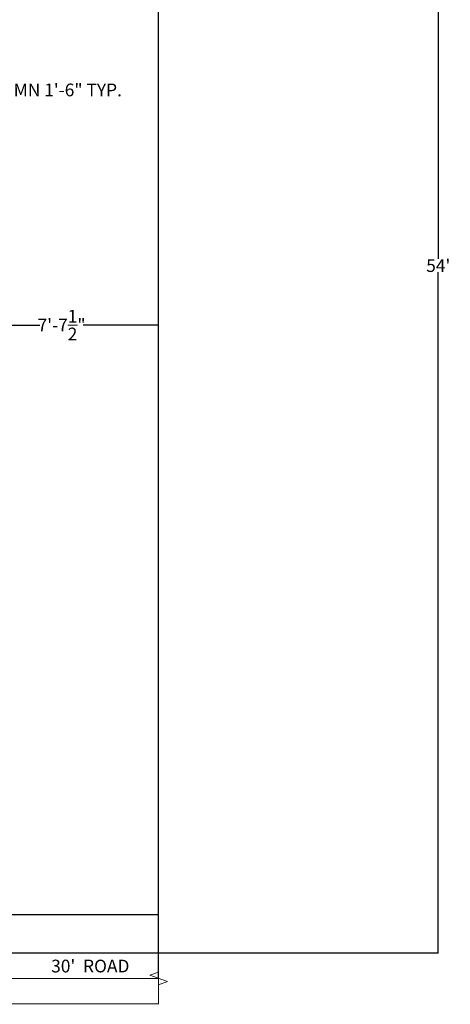
# Model space of a CAD drawing. Units: inches. Extents: x -2181 to 1225, y -80 to 4016.
# Tile 9 of 10: x 1021 to 1225, y -8 to 456. Entities that reach past the tile are written whole.
import ezdxf

# ---------------------------------------------------------------- set-up
doc = ezdxf.new("R2010")
doc.units = ezdxf.units.IN
doc.header["$MEASUREMENT"] = 0
for name, color, linetype, lineweight in [('A-ANNO-DIMS', 2, 'Continuous', 18), ('A-ANNO-TEXT', 7, 'Continuous', 18), ('C-PROP', 7, 'Continuous', 30), ('C-ROAD', 8, 'Continuous', 18)]:
    doc.layers.add(name, color=color, linetype=linetype, lineweight=lineweight)
doc.styles.get("Standard").update_dxf_attribs({"font": 'arial.ttf'})
doc.dimstyles.get("Standard").update_dxf_attribs({"dimtxt": 6, "dimasz": 0.18, "dimexe": 0.18, "dimexo": 0.0625, "dimgap": 0.09, "dimtad": 0, "dimtih": 1, "dimtoh": 1, "dimdec": 4, "dimzin": 0, "dimdsep": 46, "dimlunit": 4, "dimtxsty": 'Standard', "dimcen": 0.09, "dimadec": 0, "dimazin": 0, "dimtfac": 1, "dimtdec": 4, "dimtofl": 0, "dimtmove": 0, "dimatfit": 3, "dimfxl": 1, "dimtolj": 1, "dimtzin": 0, "dimarcsym": 0})

# ---------------------------------------------------------------- blocks, each defined once
blk = doc.blocks.new('*D25')
at = {"layer": 'A-ANNO-DIMS', "color": 0, "lineweight": -2, "transparency": 16777216}
for p, q in [((995.51, 312.49), (995.51, 312.61)), ((995.69, 312.43), (1031.04, 312.43)), ((1086.83, 312.43), (1051.49, 312.43)), ((1087.01, 312.49), (1087.01, 312.61))]:
    blk.add_line(p, q, dxfattribs=at)
at = {"layer": 'A-ANNO-DIMS', "color": 0, "transparency": 16777216}
for points in [[(995.69, 312.46), (995.69, 312.4), (995.51, 312.43)], [(1086.83, 312.46), (1086.83, 312.4), (1087.01, 312.43)]]:
    blk.add_solid(points, dxfattribs=at)
at = {"layer": 'Defpoints', "color": 0, "transparency": 16777216}
for p in [(995.51, 312.43), (1087.01, 312.43), (1087.01, 312.43)]:
    blk.add_point(p, dxfattribs=at)
at = {"layer": 'A-ANNO-DIMS', "color": 0, "transparency": 16777216, "insert": (1041.26, 312.43), "char_height": 6, "attachment_point": 5}
blk.add_mtext('\\A1;7\'-7{\\H1x;\\S1/2;}"', dxfattribs=at)
blk = doc.blocks.new('*D69')
at = {"layer": 'A-ANNO-DIMS', "color": 0, "lineweight": -2, "transparency": 16777216}
for p, q in [((808.01, 4.55), (808.01, 34.68)), ((808.19, 34.5), (937.07, 34.5)), ((1086.83, 34.5), (957.96, 34.5)), ((1087.01, 4.55), (1087.01, 34.68))]:
    blk.add_line(p, q, dxfattribs=at)
at = {"layer": 'A-ANNO-DIMS', "color": 0, "transparency": 16777216}
for points in [[(808.19, 34.53), (808.19, 34.47), (808.01, 34.5)], [(1086.83, 34.53), (1086.83, 34.47), (1087.01, 34.5)]]:
    blk.add_solid(points, dxfattribs=at)
at = {"layer": 'Defpoints', "color": 0, "transparency": 16777216}
for p in [(1087.01, 34.5), (808.01, 4.48), (1087.01, 4.48)]:
    blk.add_point(p, dxfattribs=at)
at = {"layer": 'A-ANNO-DIMS', "color": 0, "transparency": 16777216, "insert": (947.51, 34.5), "char_height": 6, "attachment_point": 5}
blk.add_mtext('\\A1;23\'-3"', dxfattribs=at)
blk = doc.blocks.new('*D73')
at = {"layer": 'A-ANNO-DIMS', "color": 0, "lineweight": -2, "transparency": 16777216}
for p, q in [((1087.08, 664.48), (1219.08, 664.48)), ((1218.9, 664.3), (1218.9, 343.63)), ((1218.9, 16.66), (1218.9, 337.34)), ((1087.08, 16.48), (1219.08, 16.48))]:
    blk.add_line(p, q, dxfattribs=at)
at = {"layer": 'A-ANNO-DIMS', "color": 0, "transparency": 16777216}
for points in [[(1218.87, 664.3), (1218.93, 664.3), (1218.9, 664.48)], [(1218.87, 16.66), (1218.93, 16.66), (1218.9, 16.48)]]:
    blk.add_solid(points, dxfattribs=at)
at = {"layer": 'Defpoints', "color": 0, "transparency": 16777216}
for p in [(1087.01, 664.48), (1218.9, 664.48), (1087.01, 16.48)]:
    blk.add_point(p, dxfattribs=at)
at = {"layer": 'A-ANNO-DIMS', "color": 0, "transparency": 16777216, "insert": (1218.9, 340.48), "char_height": 6, "attachment_point": 5}
blk.add_mtext("\\A1;54'", dxfattribs=at)
blk = doc.blocks.new('*D98')
at = {"layer": 'A-ANNO-DIMS', "color": 0, "lineweight": -2, "transparency": 16777216}
for p, q in [((977.51, 425.92), (977.51, 423.1)), ((977.69, 423.28), (995.33, 423.28)), ((995.51, 425.92), (995.51, 423.1)), ((995.51, 423.28), (995.69, 423.28))]:
    blk.add_line(p, q, dxfattribs=at)
at = {"layer": 'A-ANNO-DIMS', "color": 0, "transparency": 16777216}
for points in [[(977.69, 423.31), (977.69, 423.25), (977.51, 423.28)], [(995.33, 423.31), (995.33, 423.25), (995.51, 423.28)]]:
    blk.add_solid(points, dxfattribs=at)
at = {"layer": 'Defpoints', "color": 0, "transparency": 16777216}
for p in [(977.51, 425.98), (995.51, 425.98), (995.51, 423.28)]:
    blk.add_point(p, dxfattribs=at)
at = {"layer": 'A-ANNO-DIMS', "color": 0, "transparency": 16777216, "insert": (1033.36, 423.28), "char_height": 6, "attachment_point": 5}
blk.add_mtext('\\A1;COLUMN 1\'-6" TYP.', dxfattribs=at)

msp = doc.modelspace()

# ---------------------------------------------------------------- linework, layer by layer
at = {"layer": 'C-PROP'}
for points in [[(1087.01461, 16.48479), (1087.01461, 664.48479), (7.01461, 664.48479), (7.01461, 16.48479)], [(7.01461, 16.48479), (1087.01461, 16.48479)]]:
    msp.add_lwpolyline(points, dxfattribs=at)
at = {"layer": 'C-ROAD'}
for p, q in [((1087.01461, -7.51521), (1087.01461, 16.48479)), ((808.01461, 4.48479), (1087.01461, 4.48479))]:
    msp.add_line(p, q, dxfattribs=at)
for points in [[(1087.01461, 17.28221), (1087.01461, 7.48479), (1082.8934, 5.98479), (1091.13583, 2.98479), (1087.01461, 1.48479), (1087.01461, -7.7204)], [(7.01461, -7.51521), (1087.01461, -7.51521)]]:
    msp.add_lwpolyline(points, dxfattribs=at)

# ---------------------------------------------------------------- texts
at = {"layer": 'A-ANNO-TEXT', "insert": (1036.34969, 13.31493), "char_height": 6, "attachment_point": 1}
msp.add_mtext_dynamic_manual_height_columns("30'  ROAD", width=291.4178321, gutter_width=1, heights=[0], dxfattribs=at)

# ---------------------------------------------------------------- dimensions: what is measured, and where the dimension line sits
at = {"layer": 'A-ANNO-DIMS'}
dim = msp.add_linear_dim(base=(1218.89961, 664.48479), p1=(1087.01461, 16.48479), p2=(1087.01461, 664.48479), angle=90, dimstyle='Standard', override={"dimclrd": 0, "dimclre": 0, "dimclrt": 0}, dxfattribs=at)
dim.commit()
dim.dimension.update_dxf_attribs({"geometry": '*D73', "text_midpoint": (1218.89961, 340.48479)})
dim = msp.add_linear_dim(base=(995.51461, 423.28479), p1=(977.51461, 425.98479), p2=(995.51461, 425.98479), text='COLUMN <> TYP.', dimstyle='Standard', override={"dimdec": 1, "dimlfac": 1, "dimrnd": 0, "dimzin": 1, "dimdsep": 46, "dimlunit": 4, "dimfrac": 2}, dxfattribs=at)
dim.commit()
dim.dimension.update_dxf_attribs({"geometry": '*D98', "text_midpoint": (1033.36238, 423.28479)})
for base, p1, p2, picture, middle in [((1087.01461, 312.43008), (995.51461, 312.43008), (1087.01461, 312.43008), '*D25', (1041.26461, 312.43008)), ((1087.01461, 34.50007), (808.01461, 4.48479), (1087.01461, 4.48479), '*D69', (947.51461, 34.50007))]:
    dim = msp.add_linear_dim(base=base, p1=p1, p2=p2, dimstyle='Standard', override={"dimclrd": 0, "dimclre": 0, "dimclrt": 0}, dxfattribs=at)
    dim.commit()
    dim.dimension.update_dxf_attribs({"geometry": picture, "text_midpoint": middle})

doc.saveas('drawing.dxf')
